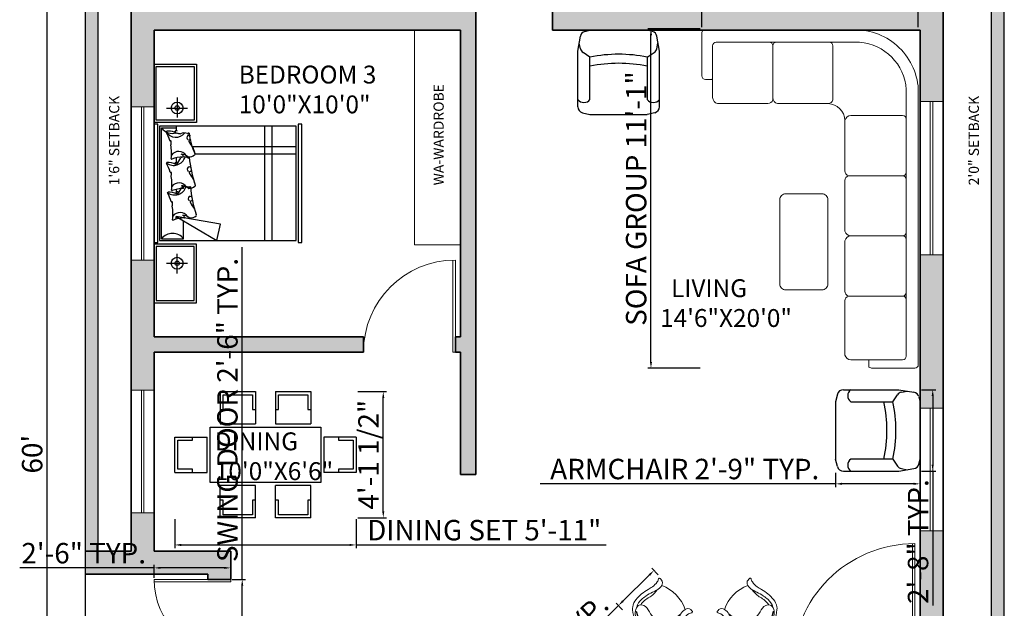
# Model space of a CAD drawing. Units: inches. Extents: x 2700 to 4052, y 1030 to 1872.
# Tile 3 of 8: x 2789 to 3175, y 1401 to 1632. Entities that reach past the tile are written whole.
import ezdxf

# ---------------------------------------------------------------- set-up
doc = ezdxf.new("R2010")
doc.units = ezdxf.units.IN
for name, color, linetype, lineweight in [('A-ANNO-DIMS', 2, 'Continuous', 13), ('A-ANNO-TEXT', 7, 'Continuous', 18), ('A-AREA-IDEN', 7, 'Continuous', 18), ('A-DOOR', 4, 'Continuous', 18), ('A-FLOR-CASE', 8, 'Continuous', 18), ('A-FURN', 8, 'Continuous', 18), ('A-GLAZ', 4, 'Continuous', 18), ('A-WALL', 7, 'Continuous', 35), ('A-WALL-PATT', 7, 'Continuous', 13), ('C-PROP', 7, 'Continuous', 25)]:
    doc.layers.add(name, color=color, linetype=linetype, lineweight=lineweight)
doc.layers.add('C-SITE-PATT', color=252, linetype='Continuous', lineweight=13, true_color=0x939598)
for name, color, linetype in [('FUR', 42, 'Continuous'), ('HA', 9, 'Continuous'), ('HBLAYER_1', 7, 'Continuous'), ('HID', 11, 'Continuous'), ('IFF-FURN-DETAIL', 250, 'Continuous'), ('NOITHAT', 21, 'Continuous'), ('SAN', 5, 'Continuous')]:
    doc.layers.add(name, color=color, linetype=linetype)
doc.styles.get("Standard").update_dxf_attribs({"font": 'arial.ttf'})
doc.dimstyles.new('ISO-25', dxfattribs={"dimtxt": 8, "dimasz": 2.5, "dimexe": 1.25, "dimexo": 0.625, "dimtad": 1, "dimdec": 1, "dimlunit": 3, "dimtxsty": 'Standard', "dimcen": 2.5, "dimclrt": 1, "dimadec": 0, "dimazin": 0, "dimtfac": 1, "dimtdec": 1, "dimtmove": 0, "dimatfit": 3, "dimfxl": 1, "dimarcsym": 0})

# ---------------------------------------------------------------- blocks, each defined once
blk = doc.blocks.new('A$C73A16738')
at = {"layer": 'FUR'}
for p, q in [((1.15, 2.389), (1.1, 2.164)), ((1.7, 2.064), (1.15, 2.389)), ((1.6, 2.364), (1.6, 2.123)), ((1.9, 2.364), (1.6, 2.364)), ((1.9, 2.364), (1.9, 0.864)), ((1.1, 2.164), (1.7, 2.064)), ((1.7, 2.099), (1.7, 2.064)), ((1.7, 1.695), (1.7, 1.735)), ((1.7, 1.268), (1.7, 1.33)), ((1.7, 0.839), (1.7, 0.904)), ((1.9, 0.864), (1.7, 0.864))]:
    blk.add_line(p, q, dxfattribs=at)
for points in [[(1.428, 2.439), (2, 2.439), (2, 3.229), (1.428, 3.229)], [(1.458, 2.469), (1.97, 2.469), (1.97, 3.199), (1.458, 3.199)], [(0, 2.414), (0, 0.814), (0.05, 0.814), (0.05, 2.414)], [(1.95, 2.414), (1.95, 0.814), (2, 0.814), (2, 2.414)], [(0.075, 0.839), (1.925, 0.839), (1.925, 2.389), (0.075, 2.389)], [(1.428, 0.789), (2, 0.789), (2, 0), (1.428, 0)], [(1.458, 0.759), (1.97, 0.759), (1.97, 0.03), (1.458, 0.03)]]:
    blk.add_lwpolyline(points, close=True, dxfattribs=at)
for centre, start, end in [((1.75, 2.481), 217.7826, 322.2174), ((1.75, 0.748), 37.7826, 105.2747)]:
    blk.add_arc(centre, 0.19, start, end, dxfattribs=at)
at = {"layer": 'HA'}
for p, q in [((0.4, 2.389), (0.4, 0.839)), ((0.5, 2.389), (0.5, 0.839)), ((1.446, 1.214), (0.075, 1.214)), ((1.477, 1.114), (0.075, 1.114))]:
    blk.add_line(p, q, dxfattribs=at)
at = {"layer": 'HID'}
for centre, radius, start, end in [((1.442, 2.042), 0.0144, 131.666, 199.4465), ((0.016, 1.539), 1.498, 4.5852, 19.4465), ((0.016, 1.539), 1.498, 16.386, 19.4465), ((1.51, 1.965), 0.117, 87.3377, 131.666), ((1.515, 2.068), 0.0144, 51.6071, 87.3377), ((1.617, 2.197), 0.15, 231.6071, 269.7845), ((1.65, 2.128), 0.12, 212.7628, 323.8922), ((1.592, 2.074), 0.0072, 92.7363, 208.2985), ((1.628, 2.093), 0.0475, 208.2985, 255.7891), ((1.569, 2.56), 0.48, 272.7363, 290.959), ((1.743, 2.106), 0.0072, 352.7248, 110.959), ((2.348, 2.029), 0.603, 172.7248, 190.2702), ((1.467, 1.966), 0.0144, 196.386, 223.7955), ((0.926, 1.551), 0.667, 29.049, 37.3823), ((1.497, 1.868), 0.0144, 282.6426, 29.049), ((2.038, 1.868), 0.288, 169.4168, 179.3085), ((1.758, 1.872), 0.0072, 179.3085, 290.689), ((1.51, 1.823), 0.0319, 112.7015, 147.1556), ((1.51, 1.821), 0.0305, 232.3565, 65.7762), ((1.503, 1.839), 0.0144, 102.6426, 112.7015), ((1.722, 1.609), 0.162, 53.8947, 162.3952), ((2.854, 0.961), 1.418, 145.8329, 150.0245), ((3.143, 2.369), 1.611, 202.7018, 202.7206), ((1.683, 1.758), 0.0288, 232.662, 339.1573), ((1.686, 1.753), 0.0072, 38.8315, 145.8329), ((1.788, 1.924), 0.192, 239.9211, 277.124), ((0.088, 1.831), 1.611, 356.4982, 357.2888), ((1.763, 1.858), 0.0072, 16.2196, 110.689), ((2.348, 2.029), 0.603, 196.2196, 208.2114), ((1.811, 1.74), 0.0072, 277.124, 28.2114), ((1.811, 1.74), 0.0072, 277.124, 28.2114), ((1.455, 1.642), 0.0144, 131.666, 199.4465), ((0.03, 1.139), 1.498, 4.5852, 19.4465), ((0.03, 1.139), 1.498, 16.386, 19.4465), ((1.524, 1.565), 0.117, 87.3377, 131.666), ((1.524, 1.653), 0.0144, 67.1663, 184.3422), ((1.529, 1.668), 0.0144, 51.6071, 87.3377), ((1.574, 1.774), 0.117, 247.1663, 295.7613), ((1.631, 1.797), 0.15, 231.6071, 269.7845), ((1.663, 1.728), 0.12, 212.7628, 323.8922), ((1.606, 1.674), 0.0072, 92.7363, 208.2985), ((1.642, 1.693), 0.0475, 208.2985, 255.7891), ((1.583, 2.161), 0.48, 272.7363, 290.959), ((1.757, 1.706), 0.0072, 352.7248, 110.959), ((2.362, 1.629), 0.603, 172.7248, 190.2702), ((1.48, 1.566), 0.0144, 196.386, 223.7955), ((0.94, 1.151), 0.667, 29.049, 37.3823), ((1.51, 1.468), 0.0144, 282.6426, 29.049), ((2.052, 1.468), 0.288, 169.4168, 179.3085), ((1.771, 1.472), 0.0072, 179.3085, 290.689), ((1.523, 1.423), 0.0319, 112.7015, 147.1556), ((1.523, 1.422), 0.0305, 232.3565, 65.7762), ((1.517, 1.44), 0.0144, 102.6426, 112.7015), ((1.736, 1.209), 0.162, 53.8947, 162.3952), ((2.867, 0.561), 1.418, 145.8329, 150.0245), ((3.156, 1.97), 1.611, 202.7018, 202.7206), ((1.697, 1.359), 0.0288, 232.662, 339.1573), ((1.7, 1.353), 0.0072, 38.8315, 145.8329), ((1.802, 1.524), 0.192, 239.9211, 277.124), ((0.102, 1.431), 1.611, 356.4982, 357.2888), ((1.776, 1.458), 0.0072, 16.2196, 110.689), ((2.362, 1.629), 0.603, 196.2196, 208.2114), ((1.825, 1.34), 0.0072, 277.124, 28.2114), ((1.825, 1.34), 0.0072, 277.124, 28.2114), ((1.46, 1.216), 0.0144, 131.666, 199.4465), ((0.688, 0.841), 0.844, 6.224, 26.0326), ((0.034, 0.713), 1.498, 16.386, 19.4465), ((1.529, 1.139), 0.117, 87.3377, 131.666), ((1.537, 1.254), 0.0144, 67.1663, 184.3422), ((1.533, 1.242), 0.0144, 51.6071, 87.3377), ((1.635, 1.371), 0.15, 231.6071, 269.7845), ((1.588, 1.374), 0.117, 247.1663, 295.7613), ((1.668, 1.302), 0.12, 212.7628, 323.8922), ((1.611, 1.248), 0.0072, 92.7363, 208.2985), ((1.646, 1.267), 0.0475, 208.2985, 255.7891), ((1.588, 1.734), 0.48, 272.7363, 290.959), ((1.762, 1.28), 0.0072, 352.7248, 110.959), ((2.367, 1.203), 0.603, 172.7248, 190.2702), ((1.485, 1.14), 0.0144, 196.386, 223.7955), ((0.945, 0.725), 0.667, 29.049, 37.3823), ((2.056, 1.042), 0.288, 169.4168, 179.3085), ((1.528, 0.997), 0.0319, 112.7015, 147.1556), ((1.528, 0.995), 0.0305, 232.3565, 65.7762), ((1.521, 1.013), 0.0144, 102.6426, 112.7015), ((1.515, 1.042), 0.0144, 282.6426, 29.049), ((1.542, 0.927), 0.0144, 67.1663, 184.3422), ((1.593, 1.048), 0.117, 247.1663, 295.7613), ((1.705, 0.84), 0.15, 29.3598, 142.4281), ((1.581, 0.528), 0.419, 73.7524, 81.4605), ((1.705, 0.927), 0.0072, 38.8315, 145.8329), ((1.776, 1.046), 0.0072, 179.3085, 290.689), ((1.781, 1.032), 0.0072, 16.2196, 110.689), ((2.367, 1.203), 0.603, 196.2196, 208.2114), ((3.161, 1.543), 1.611, 202.7018, 202.7206), ((1.702, 0.932), 0.0288, 232.662, 339.1573), ((0.106, 1.005), 1.611, 356.4982, 357.2888), ((1.806, 1.098), 0.192, 246.1093, 277.124), ((1.829, 0.914), 0.0072, 277.124, 28.2114), ((1.829, 0.914), 0.0072, 277.124, 28.2114)]:
    blk.add_arc(centre, radius, start, end, dxfattribs=at)
at = {"layer": 'SAN'}
for p, q in [((1.688, 2.835), (1.688, 2.566)), ((1.832, 2.695), (1.546, 2.695)), ((1.688, 0.454), (1.688, 0.723)), ((1.832, 0.594), (1.546, 0.594))]:
    blk.add_line(p, q, dxfattribs=at)
for centre, radius in [((1.688, 2.695), 0.08), ((1.688, 2.695), 0.03), ((1.688, 0.594), 0.08), ((1.688, 0.594), 0.03)]:
    blk.add_circle(centre, radius, dxfattribs=at)
blk = doc.blocks.new('A$C27B238C7')
at = {"layer": 'NOITHAT'}
for p, q in [((210, 810), (61, 785.2)), ((185.6, 784.9), (128.2, 796.4)), ((763.2, 810), (210, 810)), ((12.6, 740.5), (0, 690)), ((0, 120), (0, 690)), ((270, 690), (223.8, 759.3)), ((270, 690), (690, 690)), ((821.4, 764.6), (840, 690)), ((840, 120), (840, 690)), ((12.6, 69.5), (0, 120)), ((270, 120), (223.8, 50.7)), ((690, 120), (270, 120)), ((821.4, 45.4), (840, 120)), ((210, 0), (61, 24.8)), ((185.6, 25.1), (128.2, 13.6)), ((763.2, 0), (210, 0))]:
    blk.add_line(p, q, dxfattribs=at)
for centre, radius, start, end in [((70.8, 726), 60, 99.46232, 165.96376), ((173.9, 726), 60, 33.69007, 78.69007), ((645, 750), 75, 306.8699, 53.1301), ((763.2, 750), 60, 14.03624, 90), ((1608.7, 405), 1368.8, 167.98199, 192.01801), ((1698.7, 405), 1368.8, 167.98199, 192.01801), ((645, 60), 75, 306.8699, 53.1301), ((70.8, 84), 60, 194.03624, 260.53768), ((173.9, 84), 60, 281.30993, 326.30993), ((763.2, 60), 60, 270, 345.96376)]:
    blk.add_arc(centre, radius, start, end, dxfattribs=at)
blk = doc.blocks.new('A$C190E25BD')
for points in [[(2400, 82.5), (2400, 30, 0.414214), (2430, 0), (2790, 0, 0.414214), (2810, 20), (2810, 1240, 0.417206), (2320, 1800), (30, 1800, 0.414214), (0, 1770), (0, 1420, 0.162278), (10, 1390), (70, 1390)], [(2710, 1311.2, 0.371492), (2316.8, 1700), (130, 1700)], [(2710, 120), (2710, 1243.8, 0.039865), (2710, 1311.2)]]:
    blk.add_lwpolyline(points, format="xyb")
for points in [[(570, 1700), (100, 1700, 0.414214), (70, 1670), (70, 1240, 0.350781), (110, 1190), (560, 1190, 0.333333), (600, 1220), (600, 1670, 0.414214)], [(630, 1700), (1070, 1700, -0.414214), (1100, 1670), (1100, 1240, -0.350781), (1060, 1190), (640, 1190, -0.333333), (600, 1220), (600, 1670, -0.414214)], [(1570, 1700), (1130, 1700, 0.414214), (1100, 1670), (1100, 1240, 0.350781), (1140, 1190), (1560, 1190, 0.333333), (1600, 1220), (1600, 1670, 0.414214)], [(1630, 1700), (2070, 1700, -0.414214), (2100, 1670), (2100, 1240, -0.350781), (2060, 1190), (1640, 1190, -0.333333), (1600, 1220), (1600, 1670, -0.414214)], [(2710, 1060), (2710, 620, -0.414214), (2680, 590), (2250, 590, -0.350781), (2200, 630), (2200, 1050, -0.333333), (2230, 1090), (2680, 1090, -0.414214)], [(1450.6, 698), (1450.6, 998, 0.414214), (1400.6, 1048), (700.6, 1048, 0.414214), (650.6, 998), (650.6, 698, 0.414214), (700.6, 648), (1400.6, 648, 0.414214)], [(2710, 560), (2710, 120, -0.414214), (2680, 90), (2250, 90, -0.350781), (2200, 130), (2200, 550, -0.333333), (2230, 590), (2680, 590, -0.414214)]]:
    blk.add_lwpolyline(points, format="xyb", close=True)
blk.add_lwpolyline([(2702.4, 100), (2702.4, 100)])
for centre, radius, start, end in [((2052.9, 1042.9), 147.2, 2.75262, 87.24738), ((2426.3, 71.9), 28.3, 140.34955, 158.15642)]:
    blk.add_arc(centre, radius, start, end)
blk = doc.blocks.new('DIN')
at = {"layer": 'HBLAYER_1'}
for p, q in [((3337.85, 1508.09), (3337.85, 1487.39)), ((3337.85, 1508.09), (3360.51, 1508.09)), ((3339.86, 1506.07), (3358.56, 1506.07)), ((3339.86, 1496.76), (3339.86, 1506.07)), ((3358.56, 1506.07), (3358.56, 1496.76)), ((3360.51, 1508.09), (3360.51, 1487.39)), ((3373.35, 1508.09), (3396, 1508.09)), ((3373.35, 1508.09), (3373.35, 1487.39)), ((3375.3, 1506.07), (3394.05, 1506.07)), ((3375.3, 1496.76), (3375.3, 1506.07)), ((3394.05, 1506.07), (3394.05, 1496.76)), ((3396, 1508.09), (3396, 1487.39)), ((3337.85, 1496.76), (3339.86, 1496.76)), ((3358.56, 1496.76), (3360.51, 1496.76)), ((3373.35, 1496.76), (3375.3, 1496.76)), ((3394.05, 1496.76), (3396, 1496.76)), ((3331.46, 1485.44), (3402.4, 1485.44)), ((3331.46, 1449.94), (3331.46, 1485.44)), ((3337.85, 1487.39), (3360.51, 1487.39)), ((3373.35, 1487.39), (3396, 1487.39)), ((3402.4, 1485.44), (3402.4, 1449.94)), ((3308.81, 1478.98), (3329.51, 1478.98)), ((3308.81, 1456.34), (3308.81, 1478.98)), ((3320.13, 1477.03), (3320.13, 1478.98)), ((3329.51, 1456.34), (3329.51, 1478.98)), ((3425.04, 1478.98), (3404.41, 1478.98)), ((3404.41, 1478.98), (3404.41, 1456.34)), ((3413.72, 1478.98), (3413.72, 1477.03)), ((3425.04, 1478.98), (3425.04, 1456.34)), ((3310.76, 1477.03), (3320.13, 1477.03)), ((3310.76, 1458.35), (3310.76, 1477.03)), ((3413.72, 1477.03), (3423.09, 1477.03)), ((3423.09, 1477.03), (3423.09, 1458.35)), ((3320.13, 1458.35), (3310.76, 1458.35)), ((3320.13, 1456.34), (3320.13, 1458.35)), ((3423.09, 1458.35), (3413.72, 1458.35)), ((3413.72, 1458.35), (3413.72, 1456.34)), ((3308.81, 1456.34), (3329.51, 1456.34)), ((3425.04, 1456.34), (3404.41, 1456.34)), ((3402.4, 1449.94), (3331.46, 1449.94)), ((3360.51, 1447.99), (3337.85, 1447.99)), ((3337.85, 1427.29), (3337.85, 1447.99)), ((3360.51, 1427.29), (3360.51, 1447.99)), ((3396, 1447.99), (3373.35, 1447.99)), ((3373.35, 1427.29), (3373.35, 1447.99)), ((3396, 1427.29), (3396, 1447.99)), ((3339.86, 1438.62), (3337.85, 1438.62)), ((3339.86, 1429.24), (3339.86, 1438.62)), ((3360.51, 1438.62), (3358.56, 1438.62)), ((3358.56, 1438.62), (3358.56, 1429.24)), ((3375.3, 1438.62), (3373.35, 1438.62)), ((3375.3, 1429.24), (3375.3, 1438.62)), ((3396, 1438.62), (3394.05, 1438.62)), ((3394.05, 1438.62), (3394.05, 1429.24)), ((3360.51, 1427.29), (3337.85, 1427.29)), ((3358.56, 1429.24), (3339.86, 1429.24)), ((3396, 1427.29), (3373.35, 1427.29)), ((3394.05, 1429.24), (3375.3, 1429.24))]:
    blk.add_line(p, q, dxfattribs=at)
blk = doc.blocks.new('ILNG95')
for points in [[(120, 308, -0.32971), (51, 384, -0.036099), (50, 422, -0.497733), (75, 439, -0.070621), (96, 429, 0.101868), (133, 414, 0.091794), (259, 412, 0.024114), (351, 433, -0.090294), (638, 458, -0.132412), (775, 407, -0.068618), (816, 368, -0.184346), (943, 0, 1.803905)], [(120, 308, 0.138132), (244, 313, 0.001085), (325, 339, -0.034227), (462, 375, -0.033255), (567, 387, -0.137428), (727, 350, -4.561553)], [(120, 308, 0.138132), (244, 313, 0.001085), (325, 339, -0.034227), (462, 375, -0.033255), (567, 387, -0.137428), (727, 350, -4.561553)], [(235, 308, 0.064243), (394, 307, 0.04414), (433, 315, -0.118032), (643, 329, -6.296816)], [(235, 308, 0.064243), (394, 307, 0.04414), (433, 315, -0.118032), (643, 329, -6.296816)], [(639, 0, 0.078302), (612, 161, -0.233633), (633, 315, -0.28763), (710, 349, -0.317923), (875, 193, -0.032882), (900, 0, 1.140397)], [(639, 0, 0.078302), (612, 161, -0.233633), (633, 315, -0.28763), (710, 349, -0.317923), (875, 193, -0.032882), (900, 0, 1.140397)], [(120, -308, 0.32971), (51, -384, 0.036099), (50, -422, 0.497733), (75, -439, 0.070621), (96, -429, -0.101868), (133, -414, -0.091794), (259, -412, -0.024114), (351, -433, 0.090294), (638, -458, 0.132412), (775, -407, 0.068618), (816, -368, 0.184346), (943, 0, -1.803905)], [(639, 0, -0.078302), (612, -161, 0.233633), (633, -315, 0.28763), (710, -349, 0.317923), (875, -193, 0.032882), (900, 0, -1.140397)], [(639, 0, -0.078302), (612, -161, 0.233633), (633, -315, 0.28763), (710, -349, 0.317923), (875, -193, 0.032882), (900, 0, -1.140397)], [(120, -308, -0.138132), (244, -313, -0.001085), (325, -339, 0.034227), (462, -375, 0.033255), (567, -387, 0.137428), (727, -350, 4.561553)], [(120, -308, -0.138132), (244, -313, -0.001085), (325, -339, 0.034227), (462, -375, 0.033255), (567, -387, 0.137428), (727, -350, 4.561553)], [(235, -308, -0.064243), (394, -307, -0.04414), (433, -315, 0.118032), (643, -329, 6.296816)], [(235, -308, -0.064243), (394, -307, -0.04414), (433, -315, 0.118032), (643, -329, 6.296816)]]:
    blk.add_lwpolyline(points, format="xyb")
blk.add_arc((759, 1), 709, 154.3281, 205.801)
at = {"layer": 'IFF-FURN-DETAIL'}
blk.add_arc((326, -2), 549, 326.8997, 34.6691, dxfattribs=at)
blk.add_arc((326, -2), 549, 326.8997, 34.6691, dxfattribs=at)
blk = doc.blocks.new('*D20')
at = {"layer": 'A-ANNO-DIMS', "color": 0, "lineweight": -2, "transparency": 16777216}
for p, q in [((2814.04, 1821.52), (2798.4, 1821.52)), ((2799.65, 1819.02), (2799.65, 1104.02)), ((2814.04, 1101.52), (2798.4, 1101.52))]:
    blk.add_line(p, q, dxfattribs=at)
at = {"layer": 'A-ANNO-DIMS', "color": 0, "transparency": 16777216}
for points in [[(2799.23, 1819.02), (2800.06, 1819.02), (2799.65, 1821.52)], [(2799.23, 1104.02), (2800.06, 1104.02), (2799.65, 1101.52)]]:
    blk.add_solid(points, dxfattribs=at)
at = {"layer": 'Defpoints', "color": 0, "transparency": 16777216}
for p in [(2814.67, 1821.52), (2799.65, 1101.52), (2814.67, 1101.52)]:
    blk.add_point(p, dxfattribs=at)
at = {"layer": 'A-ANNO-DIMS', "color": 0, "transparency": 16777216, "insert": (2794.94, 1461.52), "char_height": 8, "attachment_point": 5, "rotation": 90}
blk.add_mtext("60'", dxfattribs=at)
blk = doc.blocks.new('DOOR-SWING-48IN')
for p, q in [((-1, 48), (-1, 0)), ((0, 48), (0, 0)), ((0, 0), (-1, 0))]:
    blk.add_line(p, q)
blk.add_arc((0, 0), 48, 90, 180)
blk = doc.blocks.new('DOOR-SWING-36IN')
for p, q in [((-1, 36), (-1, 0)), ((0, 36), (0, 0)), ((0, 0), (-1, 0))]:
    blk.add_line(p, q)
blk.add_arc((0, 0), 36, 90, 180)
blk = doc.blocks.new('DOOR-SWING-30IN')
for p, q in [((-1, 30), (-1, 0)), ((0, 30), (0, 0)), ((0, 0), (-1, 0))]:
    blk.add_line(p, q)
blk.add_arc((0, 0), 30, 90, 180)
blk = doc.blocks.new('WINDOW-48IN')
for p, q in [((-24, -4.5), (-24, 4.5)), ((24, -4.5), (24, 4.5)), ((-24, 0.5), (24, 0.5)), ((-24, -0.5), (24, -0.5))]:
    blk.add_line(p, q)
blk = doc.blocks.new('WINDOW-60IN')
for p, q in [((4.5, 30), (-4.5, 30)), ((-0.5, 30), (-0.5, -30)), ((0.5, 30), (0.5, -30)), ((4.5, -30), (-4.5, -30))]:
    blk.add_line(p, q)
blk = doc.blocks.new('*D72')
at = {"layer": 'A-ANNO-DIMS', "color": 0, "lineweight": -2, "transparency": 16777216}
for p, q in [((2876.17, 1412.52), (2876.17, 1542.6)), ((2872.29, 1412.52), (2877.42, 1412.52)), ((2876.17, 1385.02), (2876.17, 1410.02)), ((2872.29, 1382.52), (2877.42, 1382.52))]:
    blk.add_line(p, q, dxfattribs=at)
at = {"layer": 'A-ANNO-DIMS', "color": 0, "transparency": 16777216}
for points in [[(2875.75, 1410.02), (2876.59, 1410.02), (2876.17, 1412.52)], [(2875.75, 1385.02), (2876.59, 1385.02), (2876.17, 1382.52)]]:
    blk.add_solid(points, dxfattribs=at)
at = {"layer": 'Defpoints', "color": 0, "transparency": 16777216}
for p in [(2871.67, 1412.52), (2876.17, 1412.52), (2871.67, 1382.52)]:
    blk.add_point(p, dxfattribs=at)
at = {"layer": 'A-ANNO-DIMS', "color": 1, "transparency": 16777216, "insert": (2871.41, 1478.81), "char_height": 8, "attachment_point": 5, "rotation": 90}
blk.add_mtext('SWING DOOR 2\'-6" TYP.', dxfattribs=at)
blk = doc.blocks.new('*D73')
at = {"layer": 'A-ANNO-DIMS', "color": 0, "lineweight": -2, "transparency": 16777216}
for p, q in [((2841.67, 1417.02), (2789.02, 1417.02)), ((2841.67, 1413.14), (2841.67, 1418.27)), ((2869.17, 1417.02), (2844.17, 1417.02)), ((2871.67, 1413.14), (2871.67, 1418.27))]:
    blk.add_line(p, q, dxfattribs=at)
at = {"layer": 'A-ANNO-DIMS', "color": 0, "transparency": 16777216}
for points in [[(2844.17, 1417.43), (2844.17, 1416.6), (2841.67, 1417.02)], [(2869.17, 1417.43), (2869.17, 1416.6), (2871.67, 1417.02)]]:
    blk.add_solid(points, dxfattribs=at)
at = {"layer": 'Defpoints', "color": 0, "transparency": 16777216}
for p in [(2841.67, 1417.02), (2841.67, 1412.52), (2871.67, 1412.52)]:
    blk.add_point(p, dxfattribs=at)
at = {"layer": 'A-ANNO-DIMS', "color": 1, "transparency": 16777216, "insert": (2814.09, 1421.73), "char_height": 8, "attachment_point": 5}
blk.add_mtext('2\'-6" TYP.', dxfattribs=at)
blk = doc.blocks.new('*D83')
at = {"layer": 'A-ANNO-DIMS', "color": 0, "lineweight": -2, "transparency": 16777216}
for p, q in [((3039.09, 1414.33), (3036.56, 1416.89)), ((3035.66, 1414.24), (3025.31, 1404.03)), ((3023.53, 1402.27), (2973.4, 1352.84)), ((3025.17, 1400.6), (3022.65, 1403.16))]:
    blk.add_line(p, q, dxfattribs=at)
at = {"layer": 'A-ANNO-DIMS', "color": 0, "transparency": 16777216}
for points in [[(3035.37, 1414.54), (3035.95, 1413.94), (3037.44, 1416)], [(3025.01, 1404.33), (3025.6, 1403.73), (3023.53, 1402.27)]]:
    blk.add_solid(points, dxfattribs=at)
at = {"layer": 'Defpoints', "color": 0, "transparency": 16777216}
for p in [(3039.52, 1413.88), (3023.53, 1402.27), (3025.61, 1400.16)]:
    blk.add_point(p, dxfattribs=at)
at = {"layer": 'A-ANNO-DIMS', "color": 1, "transparency": 16777216, "insert": (2994.23, 1380.07), "char_height": 8, "attachment_point": 5, "rotation": 44.6051}
blk.add_mtext('1\'-7 1/2" TYP.', dxfattribs=at)
blk = doc.blocks.new('*D86')
at = {"layer": 'A-ANNO-DIMS', "color": 0, "lineweight": -2, "transparency": 16777216}
for p, q in [((3108.6, 1454.26), (3108.6, 1448.67)), ((3141.67, 1454.26), (3141.67, 1448.67)), ((3108.6, 1449.92), (2992.91, 1449.92)), ((3139.17, 1449.92), (3111.1, 1449.92))]:
    blk.add_line(p, q, dxfattribs=at)
at = {"layer": 'A-ANNO-DIMS', "color": 0, "transparency": 16777216}
for points in [[(3111.1, 1450.34), (3111.1, 1449.5), (3108.6, 1449.92)], [(3139.17, 1450.34), (3139.17, 1449.5), (3141.67, 1449.92)]]:
    blk.add_solid(points, dxfattribs=at)
at = {"layer": 'Defpoints', "color": 0, "transparency": 16777216}
for p in [(3108.6, 1454.88), (3141.67, 1454.88), (3108.6, 1449.92)]:
    blk.add_point(p, dxfattribs=at)
at = {"layer": 'A-ANNO-DIMS', "color": 1, "transparency": 16777216, "insert": (3049.5, 1454.68), "char_height": 8, "attachment_point": 5}
blk.add_mtext('ARMCHAIR 2\'-9" TYP.', dxfattribs=at)
blk = doc.blocks.new('*D87')
at = {"layer": 'A-ANNO-DIMS', "color": 0, "lineweight": -2, "transparency": 16777216}
for p, q in [((3142.29, 1486.77), (3147.88, 1486.77)), ((3146.63, 1484.27), (3146.63, 1457.38)), ((3142.29, 1454.88), (3147.88, 1454.88)), ((3146.63, 1454.88), (3146.63, 1402.23))]:
    blk.add_line(p, q, dxfattribs=at)
at = {"layer": 'A-ANNO-DIMS', "color": 0, "transparency": 16777216}
for points in [[(3146.21, 1484.27), (3147.05, 1484.27), (3146.63, 1486.77)], [(3146.21, 1457.38), (3147.05, 1457.38), (3146.63, 1454.88)]]:
    blk.add_solid(points, dxfattribs=at)
at = {"layer": 'Defpoints', "color": 0, "transparency": 16777216}
for p in [(3141.67, 1486.77), (3141.67, 1454.88), (3146.63, 1454.88)]:
    blk.add_point(p, dxfattribs=at)
at = {"layer": 'A-ANNO-DIMS', "color": 1, "transparency": 16777216, "insert": (3141.92, 1427.31), "char_height": 8, "attachment_point": 5, "rotation": 90}
blk.add_mtext('2\'-8" TYP.', dxfattribs=at)
blk = doc.blocks.new('*D90')
at = {"layer": 'A-ANNO-DIMS', "color": 0, "lineweight": -2, "transparency": 16777216}
for p, q in [((3055.57, 1627.99), (3035.02, 1627.99)), ((3036.27, 1497.66), (3036.27, 1625.49)), ((3055.57, 1495.16), (3035.02, 1495.16))]:
    blk.add_line(p, q, dxfattribs=at)
at = {"layer": 'A-ANNO-DIMS', "color": 0, "transparency": 16777216}
for points in [[(3035.86, 1625.49), (3036.69, 1625.49), (3036.27, 1627.99)], [(3035.86, 1497.66), (3036.69, 1497.66), (3036.27, 1495.16)]]:
    blk.add_solid(points, dxfattribs=at)
at = {"layer": 'Defpoints', "color": 0, "transparency": 16777216}
for p in [(3036.27, 1627.99), (3056.2, 1627.99), (3056.2, 1495.16)]:
    blk.add_point(p, dxfattribs=at)
at = {"layer": 'A-ANNO-DIMS', "color": 1, "transparency": 16777216, "insert": (3031.51, 1561.58), "char_height": 8, "attachment_point": 5, "rotation": 90}
blk.add_mtext('SOFA GROUP 11\'-1"', dxfattribs=at)
blk = doc.blocks.new('*D91')
at = {"layer": 'A-ANNO-DIMS', "color": 0, "lineweight": -2, "transparency": 16777216}
for p, q in [((3056.2, 1628.61), (3056.2, 1649.16)), ((3058.7, 1647.91), (3138.48, 1647.91)), ((3140.98, 1628.61), (3140.98, 1649.16))]:
    blk.add_line(p, q, dxfattribs=at)
at = {"layer": 'A-ANNO-DIMS', "color": 0, "transparency": 16777216}
for points in [[(3058.7, 1648.33), (3058.7, 1647.5), (3056.2, 1647.91)], [(3138.48, 1648.33), (3138.48, 1647.5), (3140.98, 1647.91)]]:
    blk.add_solid(points, dxfattribs=at)
at = {"layer": 'Defpoints', "color": 0, "transparency": 16777216}
for p in [(3140.98, 1647.91), (3056.2, 1627.99), (3140.98, 1627.99)]:
    blk.add_point(p, dxfattribs=at)
at = {"layer": 'A-ANNO-DIMS', "color": 1, "transparency": 16777216, "insert": (3098.59, 1652.55), "char_height": 8, "attachment_point": 5}
blk.add_mtext('7\'-1"', dxfattribs=at)
blk = doc.blocks.new('*D92')
at = {"layer": 'A-ANNO-DIMS', "color": 0, "lineweight": -2, "transparency": 16777216}
for p, q in [((2849.77, 1436.02), (2849.77, 1424.74)), ((2920.77, 1436.02), (2920.77, 1424.74)), ((2852.27, 1425.99), (2918.27, 1425.99)), ((2920.77, 1425.99), (3018.67, 1425.99))]:
    blk.add_line(p, q, dxfattribs=at)
at = {"layer": 'A-ANNO-DIMS', "color": 0, "transparency": 16777216}
for points in [[(2852.27, 1426.41), (2852.27, 1425.58), (2849.77, 1425.99)], [(2918.27, 1426.41), (2918.27, 1425.58), (2920.77, 1425.99)]]:
    blk.add_solid(points, dxfattribs=at)
at = {"layer": 'Defpoints', "color": 0, "transparency": 16777216}
for p in [(2849.77, 1436.64), (2920.77, 1436.64), (2920.77, 1425.99)]:
    blk.add_point(p, dxfattribs=at)
at = {"layer": 'A-ANNO-DIMS', "color": 1, "transparency": 16777216, "insert": (2970.97, 1430.75), "char_height": 8, "attachment_point": 5}
blk.add_mtext('DINING SET 5\'-11"', dxfattribs=at)
blk = doc.blocks.new('*D93')
at = {"layer": 'A-ANNO-DIMS', "color": 0, "lineweight": -2, "transparency": 16777216}
for p, q in [((2921.4, 1486), (2932.67, 1486)), ((2931.42, 1439.14), (2931.42, 1483.5)), ((2921.4, 1436.64), (2932.67, 1436.64))]:
    blk.add_line(p, q, dxfattribs=at)
at = {"layer": 'A-ANNO-DIMS', "color": 0, "transparency": 16777216}
for points in [[(2931.01, 1483.5), (2931.84, 1483.5), (2931.42, 1486)], [(2931.01, 1439.14), (2931.84, 1439.14), (2931.42, 1436.64)]]:
    blk.add_solid(points, dxfattribs=at)
at = {"layer": 'Defpoints', "color": 0, "transparency": 16777216}
for p in [(2920.77, 1486), (2931.42, 1486), (2920.77, 1436.64)]:
    blk.add_point(p, dxfattribs=at)
at = {"layer": 'A-ANNO-DIMS', "color": 1, "transparency": 16777216, "insert": (2926.66, 1461.32), "char_height": 8, "attachment_point": 5, "rotation": 90}
blk.add_mtext('4\'-1 1/2"', dxfattribs=at)

msp = doc.modelspace()

# ---------------------------------------------------------------- hatches: boundary and pattern name
at = {"layer": 'A-WALL-PATT'}
h = msp.add_hatch(color=256, dxfattribs=at)
h.dxf.hatch_style = 1
h.paths.add_polyline_path([(3150.67, 1539.52), (3141.67, 1539.52), (3141.67, 1479.52), (3150.67, 1479.52)])
h.paths.add_polyline_path([(3150.67, 1666.52), (3141.67, 1666.52), (3141.67, 1636.52), (3006.67, 1636.52), (3006.67, 1638.52), (2997.67, 1638.52), (2997.67, 1627.52), (3114.6, 1627.52, -0.035851), (3118.13, 1627.52), (3141.67, 1627.52), (3141.67, 1599.52), (3150.67, 1599.52)])
h.paths.add_polyline_path([(2841.67, 1537.52), (2832.67, 1537.52), (2832.67, 1486.52), (2841.67, 1486.52), (2841.67, 1501.52), (2923.67, 1501.52), (2923.67, 1507.52), (2841.67, 1507.52)], flags=17)
h.paths.add_polyline_path([(2841.67, 1438.52), (2832.67, 1438.52), (2832.67, 1423.52), (2814.67, 1423.52), (2814.67, 1414.52), (2862.67, 1414.52), (2862.67, 1412.52), (2871.67, 1412.52), (2871.67, 1423.52), (2841.67, 1423.52)])
h.paths.add_polyline_path([(2967.67, 1636.52), (2952.67, 1636.52), (2952.67, 1638.52), (2943.67, 1638.52), (2943.67, 1636.52), (2841.67, 1636.52), (2841.67, 1685.52), (2832.67, 1685.52), (2832.67, 1597.52), (2841.67, 1597.52), (2841.67, 1627.52), (2961.67, 1627.52), (2961.67, 1507.52), (2959.67, 1507.52), (2959.67, 1501.52), (2961.67, 1501.52), (2961.67, 1453.52), (2967.67, 1453.52)])
h.paths.add_polyline_path([(2970.67, 1756.52), (3109.67, 1756.52), (3109.67, 1762.52), (3060.67, 1762.52), (3060.67, 1812.52), (3141.67, 1812.52), (3141.67, 1799.52), (3150.67, 1799.52), (3150.67, 1821.52), (3042.67, 1821.52), (3042.67, 1812.52), (3054.67, 1812.52), (3054.67, 1762.52), (2970.67, 1762.52), (2970.67, 1764.52), (2961.67, 1764.52), (2961.67, 1686.52), (2943.67, 1686.52), (2943.67, 1674.52), (2952.67, 1674.52), (2952.67, 1677.52), (2997.67, 1677.52), (2997.67, 1674.52), (3006.67, 1674.52), (3006.67, 1686.52), (2970.67, 1686.52)])
h.paths.add_polyline_path([(3150.67, 1775.52), (3141.67, 1775.52), (3141.67, 1762.52), (3139.67, 1762.52), (3139.67, 1756.52), (3141.67, 1756.52), (3141.67, 1726.52), (3150.67, 1726.52)], flags=17)
h.paths.add_polyline_path([(3018.67, 1821.52), (2832.67, 1821.52), (2832.67, 1745.52), (2841.67, 1745.52), (2841.67, 1812.52), (2961.67, 1812.52), (2961.67, 1794.52), (2970.67, 1794.52), (2970.67, 1812.52), (3018.67, 1812.52)])
h = msp.add_hatch(color=256, dxfattribs=at)
h.dxf.hatch_style = 1
h.paths.add_polyline_path([(2814.67, 1264.52), (2814.67, 1168.52), (2955.67, 1168.52), (2955.67, 1177.52), (2823.67, 1177.52), (2823.67, 1255.52), (2897.67, 1255.52), (2897.67, 1264.52), (2871.67, 1264.52), (2871.67, 1310.49), (2862.67, 1310.49), (2862.67, 1304.37), (2862.67, 1264.52)])
h.paths.add_polyline_path([(2945.67, 1255.52), (2986.67, 1255.52), (2986.67, 1264.52), (2980.67, 1264.52), (2980.67, 1324.52), (3028.67, 1324.52), (3028.67, 1264.52), (3022.67, 1264.52), (3022.67, 1255.52), (3037.67, 1255.52), (3037.67, 1378.52), (3040.67, 1378.52), (3040.67, 1387.52), (3022.67, 1387.52), (3022.67, 1381.52), (3028.67, 1381.52), (3028.67, 1333.52), (2980.67, 1333.52), (2980.67, 1381.52), (2986.67, 1381.52), (2986.67, 1387.52), (2971.67, 1387.52), (2971.67, 1264.52), (2945.67, 1264.52)])
h.paths.add_polyline_path([(2871.67, 1358.49), (2871.67, 1382.52), (2862.67, 1382.52), (2862.67, 1358.49)])
h.paths.add_polyline_path([(3091.67, 1387.52), (3088.67, 1387.52), (3088.67, 1378.52), (3091.67, 1378.52)])
h.paths.add_polyline_path([(3141.67, 1300.52), (3150.67, 1300.52), (3150.67, 1431.52), (3141.67, 1431.52), (3141.67, 1387.52), (3139.67, 1387.52), (3139.67, 1378.52), (3141.67, 1378.52)])
h.paths.add_polyline_path([(2830.28, 1565.14), (2830.28, 1604.05), (2822.03, 1604.05), (2822.03, 1565.14)], flags=9)
h.paths.add_polyline_path([(2957.35, 1565.68), (2957.35, 1611.46), (2949.11, 1611.46), (2949.11, 1565.68)], flags=9)
h.paths.add_polyline_path([(2983.54, 1697.89), (2983.54, 1743.66), (2975.29, 1743.66), (2975.29, 1697.89)], flags=9)
h.paths.add_polyline_path([(2879.08, 1800.61), (2924.85, 1800.61), (2924.85, 1808.85), (2879.08, 1808.85)], flags=9)
h.paths.add_polyline_path([(2815.49, 1361.72), (2864.45, 1361.72), (2864.45, 1388.34), (2815.49, 1388.34)], flags=9)
h.paths.add_polyline_path([(2904.6, 1318.27), (2953.91, 1318.27), (2953.91, 1344.89), (2904.6, 1344.89)], flags=9)
h.paths.add_polyline_path([(3036.9, 1507.34), (3091.04, 1507.34), (3091.04, 1533.96), (3036.9, 1533.96)], flags=9)
h.paths.add_polyline_path([(2990.4, 1774.23), (3040.41, 1774.23), (3040.41, 1800.84), (2990.4, 1800.84)], flags=9)
h.paths.add_polyline_path([(3076.88, 1774.23), (3126.96, 1774.23), (3126.96, 1800.84), (3076.88, 1800.84)], flags=9)
h.paths.add_polyline_path([(3036.9, 1664.37), (3100.88, 1664.37), (3100.88, 1690.98), (3036.9, 1690.98)], flags=9)
h.paths.add_polyline_path([(2871.85, 1747.79), (2935.82, 1747.79), (2935.82, 1774.41), (2871.85, 1774.41)], flags=9)
h.paths.add_polyline_path([(2871.85, 1590.97), (2935.82, 1590.97), (2935.82, 1617.58), (2871.85, 1617.58)], flags=9)
h.paths.add_polyline_path([(2862.5, 1447.4), (2911.46, 1447.4), (2911.46, 1474.01), (2862.5, 1474.01)], flags=9)
at = {"layer": 'C-SITE-PATT'}
h = msp.add_hatch(color=256, dxfattribs=at)
h.dxf.hatch_style = 1
h.paths.add_polyline_path([(2819.67, 1821.52), (2814.67, 1821.52), (2814.67, 1423.52), (2819.67, 1423.52)])
h.paths.add_polyline_path([(3037.67, 1108.52), (2819.67, 1108.52), (2819.67, 1168.52), (2814.67, 1168.52), (2814.67, 1101.52), (3037.67, 1101.52)])
h.paths.add_polyline_path([(3174.67, 1821.52), (3169.67, 1821.52), (3169.67, 1108.52), (3157.67, 1108.52), (3157.67, 1101.52), (3174.67, 1101.52)])

# ---------------------------------------------------------------- linework, layer by layer
at = {"layer": 'A-FLOR-CASE'}
for p in [(2943.67, 1627.52), (2961.67, 1543.52)]:
    msp.add_line(p, (2943.67, 1543.52), dxfattribs=at)
at = {"layer": 'A-WALL'}
for p, q in [((2832.67, 1821.52), (2832.67, 1423.52)), ((3150.67, 1300.52), (3150.67, 1821.52)), ((2967.67, 1636.52), (2967.67, 1453.52)), ((2997.67, 1638.52), (2997.67, 1627.52)), ((2961.67, 1627.52), (2841.67, 1627.52)), ((2841.67, 1627.52), (2841.67, 1507.52)), ((2961.67, 1627.52), (2961.67, 1507.52)), ((3141.67, 1627.52), (2997.67, 1627.52)), ((3141.67, 1387.52), (3141.67, 1627.52)), ((2923.67, 1507.52), (2841.67, 1507.52)), ((2923.67, 1507.52), (2923.67, 1501.52)), ((2961.67, 1507.52), (2959.67, 1507.52)), ((2959.67, 1507.52), (2959.67, 1501.52)), ((2923.67, 1501.52), (2841.67, 1501.52)), ((2841.67, 1501.52), (2841.67, 1423.52)), ((2961.67, 1501.52), (2959.67, 1501.52)), ((2961.67, 1501.52), (2961.67, 1453.52)), ((2967.67, 1453.52), (2961.67, 1453.52)), ((2832.67, 1423.52), (2814.67, 1423.52)), ((2871.67, 1423.52), (2841.67, 1423.52)), ((2871.67, 1412.52), (2871.67, 1423.52)), ((2862.67, 1414.52), (2814.67, 1414.52)), ((2862.67, 1412.52), (2862.67, 1414.52)), ((2871.67, 1412.52), (2862.67, 1412.52))]:
    msp.add_line(p, q, dxfattribs=at)
at = {"layer": 'C-PROP'}
for p, q in [((2819.67, 1821.52), (2819.67, 1423.52)), ((3169.67, 1108.52), (3169.67, 1821.52))]:
    msp.add_line(p, q, dxfattribs=at)
msp.add_lwpolyline([(3157.67, 1101.52), (3174.67, 1101.52), (3174.67, 1821.52), (2814.67, 1821.52), (2814.67, 1101.52), (3037.67, 1101.52)], dxfattribs=at)

# ---------------------------------------------------------------- block references
at = {"layer": 'A-DOOR'}
for name, p in [('DOOR-SWING-36IN', (2959.67, 1501.52)), ('DOOR-SWING-48IN', (3139.67, 1378.52))]:
    msp.add_blockref(name, p, dxfattribs=at)
at = {"layer": 'A-DOOR', "rotation": 90.00000000000067}
msp.add_blockref('DOOR-SWING-30IN', (2871.67, 1412.52), dxfattribs=at)
at = {"layer": 'A-FURN'}
for name, p, xscale, yscale, zscale, rotation in [('A$C27B238C7', (3007.67, 1627.52), 0.0393701, 0.0393701, 0.0393701, 270), ('A$C190E25BD', (3056.2, 1495.16), -0.0471007408212362, 0.0471007408212362, 0.0471007408212362, 270), ('A$C73A16738', (2899.51, 1614.21), 28.92215291203286, 28.92215291203286, 28.92215291203286, 180), ('A$C27B238C7', (3141.67, 1486.77), 0.0393701, 0.0393701, 0.0393701, 180), ('ILNG95', (3046.88, 1407.22), 0.0212192471586889, 0.0212192471586889, 0.0212192471586889, 224.6051083961163), ('ILNG95', (3067.81, 1407.22), -0.0212192471586889, 0.0212192471586889, 0.0212192471586889, 135.3948916038836)]:
    msp.add_blockref(name, p, dxfattribs=dict(at, xscale=xscale, yscale=yscale, zscale=zscale, rotation=rotation))
at = {"layer": 'A-FURN', "xscale": 0.6108839328517579, "yscale": 0.6108839328517579, "zscale": 0.6108839328517579}
msp.add_blockref('DIN', (828.47, 564.73), dxfattribs=at)
at = {"layer": 'A-GLAZ'}
for p in [(2837.17, 1567.52), (3146.17, 1569.52)]:
    msp.add_blockref('WINDOW-60IN', p, dxfattribs=at)
for p, rotation in [((2837.17, 1462.52), 90.00000000000595), ((3146.17, 1455.52), 90.00000000000487)]:
    msp.add_blockref('WINDOW-48IN', p, dxfattribs=dict(at, rotation=rotation))

# ---------------------------------------------------------------- texts
at = {"layer": 'A-ANNO-TEXT', "char_height": 4, "attachment_point": 1, "rotation": 90}
for s, width, insert in [('WA-WARDROBE', 29.5334, (2951.1, 1566.75)), ('1\'6" SETBACK', 45.8842, (2824.02, 1566.75)), ('2\'0" SETBACK', 41.5432, (3160.72, 1566.75))]:
    msp.add_mtext_dynamic_manual_height_columns(s, width=width, gutter_width=12.5, heights=[0], dxfattribs=dict(at, insert=insert))
at = {"layer": 'A-AREA-IDEN', "char_height": 7, "attachment_point": 1}
for s, insert in [('{\\fTimes New Roman|b0|i0|c0|p18;BEDROOM 3\\P10\'0"X10\'0"}', (2874.81, 1613.62)), ('{\\fTimes New Roman|b0|i0|c0|p18;  LIVING\\P14\'6"X20\'0"}', (3039.86, 1530)), ('{\\fTimes New Roman|b0|i0|c0|p18;DINING\\P10\'0"X6\'6"}', (2865.46, 1470.05))]:
    msp.add_mtext_dynamic_manual_height_columns(s, width=61.0557, gutter_width=12.5, heights=[0], dxfattribs=dict(at, insert=insert))

# ---------------------------------------------------------------- dimensions: what is measured, and where the dimension line sits
at = {"layer": 'A-ANNO-DIMS'}
for base, p1, p2, override, picture, middle in [((2799.65, 1101.52), (2814.67, 1821.52), (2814.67, 1101.52), {"dimclrd": 0, "dimclre": 0, "dimclrt": 0}, '*D20', (2794.94, 1461.52)), ((2931.42, 1486), (2920.77, 1436.64), (2920.77, 1486), {"dimdec": 1, "dimlfac": 1, "dimrnd": 0, "dimzin": 1, "dimdsep": 46, "dimlunit": 4, "dimfrac": 2}, '*D93', (2926.66, 1461.32))]:
    dim = msp.add_linear_dim(base=base, p1=p1, p2=p2, angle=90, dimstyle='ISO-25', override=override, dxfattribs=at)
    dim.commit()
    dim.dimension.update_dxf_attribs({"geometry": picture, "text_midpoint": middle})
dim = msp.add_linear_dim(base=(3140.98, 1647.91), p1=(3056.2, 1627.99), p2=(3140.98, 1627.99), dimstyle='ISO-25', override={"dimdec": 1, "dimlfac": 1, "dimrnd": 0, "dimzin": 1, "dimdsep": 46, "dimlunit": 4, "dimfrac": 2}, dxfattribs=at)
dim.commit()
dim.dimension.update_dxf_attribs({"geometry": '*D91', "text_midpoint": (3098.59, 1652.55)})
for base, p1, p2, angle, text, picture, middle in [((3036.27, 1627.99), (3056.2, 1495.16), (3056.2, 1627.99), 90, 'SOFA GROUP <>', '*D90', (3031.51, 1561.58)), ((2876.17, 1412.52), (2871.67, 1382.52), (2871.67, 1412.52), 90, 'SWING DOOR <> TYP.', '*D72', (2871.41, 1478.81)), ((3146.63, 1454.88), (3141.67, 1486.77), (3141.67, 1454.88), 270, '<> TYP.', '*D87', (3141.92, 1427.31)), ((3108.6, 1449.92), (3141.67, 1454.88), (3108.6, 1454.88), 180, 'ARMCHAIR <> TYP.', '*D86', (3049.5, 1454.68)), ((2841.67, 1417.02), (2871.67, 1412.52), (2841.67, 1412.52), 180, '<> TYP.', '*D73', (2814.09, 1421.73)), ((3023.53, 1402.27), (3039.52, 1413.88), (3025.61, 1400.16), 224.6051, '<> TYP.', '*D83', (2994.23, 1380.07))]:
    dim = msp.add_linear_dim(base=base, p1=p1, p2=p2, angle=angle, text=text, dimstyle='ISO-25', override={"dimdec": 1, "dimlfac": 1, "dimrnd": 0, "dimzin": 1, "dimdsep": 46, "dimlunit": 4, "dimfrac": 2}, dxfattribs=at)
    dim.commit()
    dim.dimension.update_dxf_attribs({"geometry": picture, "text_midpoint": middle})
dim = msp.add_linear_dim(base=(2920.77, 1425.99), p1=(2849.77, 1436.64), p2=(2920.77, 1436.64), text='DINING SET <>', dimstyle='ISO-25', override={"dimdec": 1, "dimlfac": 1, "dimrnd": 0, "dimzin": 1, "dimdsep": 46, "dimlunit": 4, "dimfrac": 2}, dxfattribs=at)
dim.commit()
dim.dimension.update_dxf_attribs({"geometry": '*D92', "text_midpoint": (2970.97, 1430.75)})

doc.saveas('drawing.dxf')
